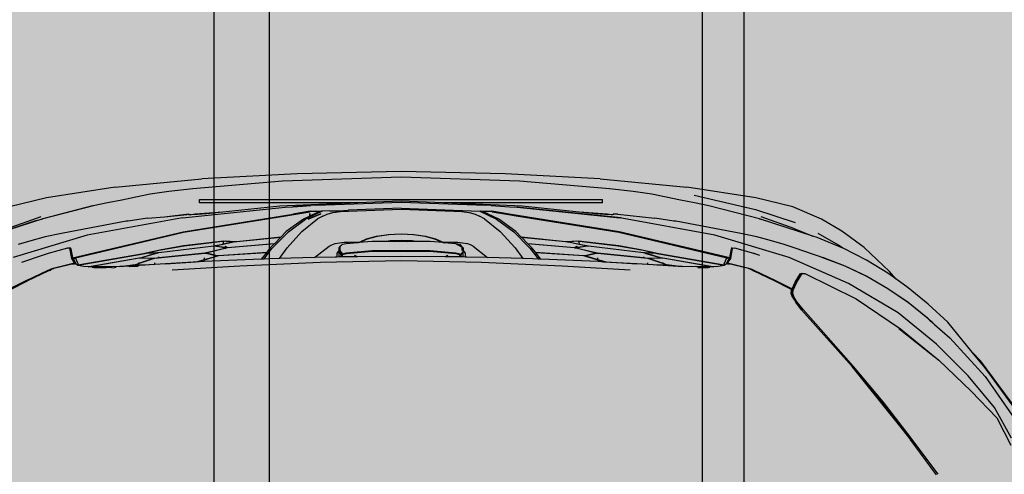
# Model space of a CAD drawing. Units: inches. Extents: x 1884 to 2398, y 474 to 1488.
# Tile 29 of 39: x 2306 to 2356, y 737 to 761. Entities that reach past the tile are written whole.
import ezdxf

# ---------------------------------------------------------------- set-up
doc = ezdxf.new("R2010")
doc.units = ezdxf.units.IN
doc.header["$MEASUREMENT"] = 0
doc.layers.get('0').update_dxf_attribs({"color": 250})
doc.layers.add('A-ANNO-DIMS', color=2, linetype='Continuous', lineweight=18)
doc.layers.add('C-VEHI', color=8, linetype='Continuous', lineweight=18)
doc.layers.add('Edges', color=250, linetype='Continuous')
doc.layers.add('L-PVMT-PATT', color=9, linetype='Continuous', lineweight=13, true_color=0xc7c8ca)
doc.styles.get("Standard").update_dxf_attribs({"font": 'arial.ttf'})
doc.dimstyles.get("Standard").update_dxf_attribs({"dimtxt": 7, "dimasz": 0.18, "dimexe": 0.18, "dimexo": 0.0625, "dimgap": 0.09, "dimtad": 0, "dimtih": 1, "dimtoh": 1, "dimzin": 0, "dimdsep": 46, "dimlunit": 3, "dimtxsty": 'Standard', "dimcen": 0.09, "dimadec": 0, "dimazin": 0, "dimtfac": 1, "dimtofl": 0, "dimtmove": 0, "dimatfit": 3, "dimfxl": 1, "dimtolj": 1, "dimtzin": 0, "dimarcsym": 0})

# ---------------------------------------------------------------- blocks, each defined once
blk = doc.blocks.new('Nissan Qashqai pl')
at = {"layer": 'Edges'}
for p, q in [((7.6024, 12.7221), (7.5387, 12.6759)), ((7.5946, 12.718), (7.5304, 12.6704)), ((7.5501, 12.6757), (7.6051, 12.7139)), ((7.6295, 12.7097), (7.59, 12.6877)), ((7.6032, 12.6908), (7.6386, 12.7089)), ((7.59, 12.6877), (7.5492, 12.654)), ((7.5687, 12.6579), (7.6032, 12.6908)), ((7.5501, 12.6757), (7.5001, 12.6302)), ((7.5387, 12.6759), (7.5184, 12.6591)), ((7.5184, 12.6591), (7.5304, 12.6704)), ((7.5184, 12.6591), (7.4801, 12.6274)), ((7.5289, 12.6158), (7.5687, 12.6579)), ((7.5492, 12.654), (7.531, 12.6359)), ((7.4827, 12.6103), (7.5001, 12.6302)), ((7.531, 12.6359), (7.5081, 12.6131)), ((7.531, 12.6359), (7.5301, 12.6353)), ((7.4801, 12.6274), (7.4565, 12.6023)), ((7.5081, 12.6131), (7.4679, 12.5634)), ((7.4744, 12.6015), (7.4804, 12.6079)), ((7.4762, 12.6028), (7.478, 12.6049)), ((7.4804, 12.6079), (7.478, 12.6049)), ((7.478, 12.6049), (7.479, 12.6061)), ((7.479, 12.6061), (7.4815, 12.6089)), ((7.479, 12.6061), (7.4801, 12.6074)), ((7.4801, 12.6074), (7.4804, 12.6079)), ((7.4804, 12.6079), (7.4807, 12.6082)), ((7.4804, 12.6079), (7.4804, 12.6079)), ((7.4807, 12.6082), (7.4821, 12.6097)), ((7.4815, 12.6089), (7.4821, 12.6097)), ((7.4821, 12.6097), (7.4827, 12.6103)), ((7.4882, 12.5645), (7.5243, 12.6101)), ((7.4884, 12.5664), (7.5289, 12.6158)), ((7.5243, 12.6101), (7.5286, 12.6146)), ((7.676, 12.6152), (7.6296, 12.5803)), ((7.6769, 12.6129), (7.6306, 12.5791)), ((7.4565, 12.6023), (7.4354, 12.5766)), ((7.4542, 12.5765), (7.4744, 12.6015)), ((7.475, 12.6016), (7.4549, 12.5767)), ((7.4762, 12.6028), (7.475, 12.6016)), ((7.4752, 12.6016), (7.4762, 12.6028)), ((7.6296, 12.5803), (7.5827, 12.5441)), ((7.6301, 12.5787), (7.618, 12.5691)), ((7.6306, 12.5791), (7.6301, 12.5787)), ((7.4354, 12.5766), (7.4239, 12.5604)), ((7.4363, 12.5502), (7.4542, 12.5765)), ((7.4549, 12.5767), (7.4369, 12.5504)), ((7.4498, 12.5093), (7.4884, 12.5664)), ((7.618, 12.5691), (7.5829, 12.5411)), ((7.618, 12.5691), (7.584, 12.5429)), ((7.4239, 12.5604), (7.4147, 12.5524)), ((7.4239, 12.5604), (7.4166, 12.5503)), ((7.4679, 12.5634), (7.4302, 12.4993)), ((7.4147, 12.5524), (7.3837, 12.5197)), ((7.4166, 12.5503), (7.3997, 12.5227)), ((7.4205, 12.5229), (7.4363, 12.5502)), ((7.4369, 12.5504), (7.4211, 12.5232)), ((7.5827, 12.5441), (7.5369, 12.5057)), ((7.584, 12.5429), (7.5568, 12.5201)), ((7.5829, 12.5411), (7.5568, 12.5201)), ((7.3837, 12.5197), (7.3624, 12.4907)), ((7.3997, 12.5227), (7.3845, 12.4925)), ((7.4071, 12.4948), (7.4205, 12.5229)), ((7.4211, 12.5232), (7.4078, 12.4951)), ((7.5568, 12.5201), (7.5371, 12.5042)), ((7.4172, 12.4431), (7.4498, 12.5093)), ((7.5369, 12.5057), (7.4635, 12.4408)), ((7.4638, 12.439), (7.5371, 12.5042)), ((7.3624, 12.4907), (7.347, 12.4644)), ((7.3843, 12.492), (7.3707, 12.4592)), ((7.3843, 12.492), (7.3805, 12.4866)), ((7.3845, 12.4925), (7.3843, 12.492)), ((7.3962, 12.466), (7.4071, 12.4948)), ((7.4302, 12.4993), (7.3963, 12.4227)), ((7.4078, 12.4951), (7.3969, 12.4665)), ((7.3805, 12.4866), (7.3655, 12.4604)), ((7.347, 12.4644), (7.3309, 12.4276)), ((7.3965, 12.4655), (7.3951, 12.462)), ((7.3965, 12.4655), (7.3962, 12.466)), ((7.3969, 12.4665), (7.3965, 12.4655)), ((7.3968, 12.4649), (7.3967, 12.4651)), ((7.3688, 12.4532), (7.3467, 12.3846)), ((7.3596, 12.4302), (7.3688, 12.4532)), ((7.3707, 12.4592), (7.3688, 12.4532)), ((7.3925, 12.4542), (7.3845, 12.4306)), ((7.3938, 12.4583), (7.3925, 12.4542)), ((7.3951, 12.462), (7.3938, 12.4583)), ((7.4167, 12.4393), (7.4169, 12.4406)), ((7.4167, 12.4393), (7.4172, 12.4395)), ((7.417, 12.4377), (7.4167, 12.4393)), ((7.4169, 12.4412), (7.4172, 12.4431)), ((7.4169, 12.4406), (7.4172, 12.4423)), ((7.4169, 12.4406), (7.4169, 12.4412)), ((7.4169, 12.4398), (7.4169, 12.4406)), ((7.4282, 12.4328), (7.4169, 12.4398)), ((7.4172, 12.4395), (7.4169, 12.4398)), ((7.4172, 12.4423), (7.4174, 12.4429)), ((7.4183, 12.4382), (7.4172, 12.4395)), ((7.4175, 12.4429), (7.4174, 12.4429)), ((7.4635, 12.4408), (7.4541, 12.4333)), ((7.4638, 12.439), (7.4541, 12.4313)), ((7.3309, 12.4276), (7.3193, 12.3797)), ((7.3345, 12.3793), (7.3514, 12.4308)), ((7.3596, 12.4302), (7.344, 12.3869)), ((7.3845, 12.4306), (7.3799, 12.4164)), ((7.4283, 12.4307), (7.417, 12.4377)), ((7.4183, 12.4382), (7.4296, 12.4312)), ((7.4255, 12.4044), (7.4367, 12.4268)), ((7.4387, 12.428), (7.4282, 12.4328)), ((7.4359, 12.4272), (7.4283, 12.4307)), ((7.4383, 12.4272), (7.4296, 12.4312)), ((7.4367, 12.4268), (7.4359, 12.4272)), ((7.4378, 12.4261), (7.4365, 12.4235)), ((7.4367, 12.4268), (7.4383, 12.4272)), ((7.4379, 12.4263), (7.4378, 12.4261)), ((7.4379, 12.4263), (7.4383, 12.4272)), ((7.4379, 12.4263), (7.4389, 12.4269)), ((7.4384, 12.426), (7.4379, 12.4263)), ((7.4384, 12.426), (7.438, 12.4251)), ((7.4383, 12.4272), (7.4389, 12.4269)), ((7.4389, 12.4269), (7.4384, 12.426)), ((7.4387, 12.4259), (7.4384, 12.426)), ((7.4431, 12.4276), (7.4387, 12.428)), ((7.443, 12.4254), (7.4387, 12.4259)), ((7.44, 12.4264), (7.4389, 12.4269)), ((7.44, 12.4264), (7.4442, 12.4258)), ((7.4477, 12.427), (7.443, 12.4254)), ((7.4479, 12.4293), (7.4431, 12.4276)), ((7.4442, 12.4258), (7.4477, 12.427)), ((7.4477, 12.427), (7.4541, 12.4313)), ((7.4541, 12.4333), (7.4479, 12.4293)), ((7.3963, 12.4227), (7.3676, 12.3269)), ((7.3799, 12.4164), (7.375, 12.4)), ((7.4365, 12.4235), (7.4267, 12.4041)), ((7.4365, 12.4235), (7.4365, 12.4235)), ((7.4131, 12.3783), (7.4255, 12.4044)), ((7.4267, 12.4041), (7.4139, 12.3778)), ((7.3467, 12.3846), (7.3489, 12.3925)), ((7.375, 12.4), (7.3699, 12.3813)), ((7.3193, 12.3797), (7.3059, 12.291)), ((7.3161, 12.3001), (7.3345, 12.3793)), ((7.3467, 12.3846), (7.33, 12.3192)), ((7.3699, 12.3813), (7.3653, 12.3604)), ((7.3913, 12.3774), (7.3844, 12.3526)), ((7.3913, 12.3774), (7.3914, 12.3775)), ((7.3925, 12.3813), (7.3914, 12.3775)), ((7.3937, 12.3851), (7.3925, 12.3813)), ((7.4115, 12.3746), (7.4131, 12.3783)), ((7.4139, 12.3778), (7.4122, 12.3742)), ((7.4133, 12.3759), (7.4142, 12.3776)), ((7.4033, 12.3435), (7.4101, 12.3708)), ((7.4108, 12.3703), (7.4042, 12.3435)), ((7.4101, 12.3708), (7.4115, 12.3746)), ((7.4122, 12.3742), (7.4108, 12.3703)), ((7.3653, 12.3604), (7.3497, 12.2767)), ((7.3841, 12.3485), (7.3844, 12.3526)), ((7.3971, 12.3461), (7.3635, 12.2033)), ((7.364, 12.2029), (7.3968, 12.3424)), ((7.3846, 12.3495), (7.3841, 12.3485)), ((7.3841, 12.3485), (7.3853, 12.3483)), ((7.3846, 12.3495), (7.3976, 12.347)), ((7.3971, 12.3461), (7.3853, 12.3483)), ((7.3916, 12.2547), (7.4062, 12.3389)), ((7.4065, 12.3392), (7.3917, 12.2547)), ((7.3968, 12.3424), (7.398, 12.3449)), ((7.4046, 12.3389), (7.3968, 12.3424)), ((7.3983, 12.3458), (7.3971, 12.3461)), ((7.3976, 12.347), (7.4026, 12.3439)), ((7.398, 12.3449), (7.3999, 12.344)), ((7.398, 12.3449), (7.4012, 12.3441)), ((7.4012, 12.3441), (7.3983, 12.3458)), ((7.3999, 12.344), (7.4051, 12.3415)), ((7.3999, 12.344), (7.4048, 12.3417)), ((7.4033, 12.3427), (7.4012, 12.3441)), ((7.4012, 12.3441), (7.4015, 12.344)), ((7.4015, 12.344), (7.4028, 12.3437)), ((7.4026, 12.3439), (7.4033, 12.3435)), ((7.4033, 12.3435), (7.4042, 12.3422)), ((7.4042, 12.3422), (7.4033, 12.3427)), ((7.4042, 12.3435), (7.404, 12.3429)), ((7.404, 12.3429), (7.4043, 12.3428)), ((7.404, 12.3429), (7.4043, 12.3425)), ((7.4041, 12.3435), (7.4042, 12.3435)), ((7.4042, 12.3435), (7.4045, 12.3434)), ((7.4042, 12.3422), (7.4043, 12.3425)), ((7.4044, 12.3422), (7.4042, 12.3422)), ((7.4043, 12.3428), (7.4045, 12.3434)), ((7.4043, 12.3428), (7.4046, 12.3425)), ((7.4043, 12.3425), (7.4043, 12.3428)), ((7.4043, 12.3425), (7.4044, 12.3422)), ((7.4044, 12.3422), (7.4046, 12.3419)), ((7.4046, 12.3422), (7.4044, 12.3422)), ((7.4045, 12.3434), (7.405, 12.3456)), ((7.4045, 12.3434), (7.4048, 12.3433)), ((7.4046, 12.3425), (7.4047, 12.3424)), ((7.4047, 12.3424), (7.4046, 12.3422)), ((7.4046, 12.3422), (7.4046, 12.3419)), ((7.4048, 12.3422), (7.4046, 12.3422)), ((7.4046, 12.3419), (7.405, 12.3419)), ((7.4048, 12.3417), (7.4046, 12.3419)), ((7.4046, 12.3389), (7.4062, 12.3389)), ((7.4047, 12.3424), (7.4048, 12.3422)), ((7.4048, 12.3422), (7.405, 12.3419)), ((7.4048, 12.3417), (7.4052, 12.3416)), ((7.4051, 12.3415), (7.4048, 12.3417)), ((7.405, 12.3419), (7.4052, 12.3416)), ((7.4051, 12.3415), (7.4052, 12.3415)), ((7.4052, 12.3416), (7.4052, 12.3415)), ((7.4052, 12.3415), (7.4063, 12.3395)), ((7.4062, 12.3389), (7.4063, 12.3395)), ((7.4063, 12.3395), (7.4065, 12.3392)), ((7.4065, 12.3392), (7.4066, 12.3389)), ((7.4066, 12.3389), (7.408, 12.3313)), ((7.3676, 12.3269), (7.3455, 12.2042)), ((7.3971, 12.2599), (7.4083, 12.3258)), ((7.4084, 12.3244), (7.3975, 12.2599)), ((7.408, 12.3313), (7.4083, 12.3258)), ((7.4083, 12.3258), (7.4084, 12.3244)), ((7.4084, 12.3244), (7.4087, 12.3195)), ((7.33, 12.3192), (7.3261, 12.3009)), ((7.4087, 12.3195), (7.4087, 12.3037)), ((7.4092, 12.3184), (7.4091, 12.3206)), ((7.4092, 12.305), (7.4092, 12.3184)), ((7.3261, 12.3009), (7.3223, 12.2825)), ((7.4087, 12.3037), (7.4081, 12.2848)), ((7.2951, 12.1791), (7.3059, 12.291)), ((7.3223, 12.2825), (7.3186, 12.2641)), ((7.3494, 12.2741), (7.3457, 12.2495)), ((7.3498, 12.2768), (7.3494, 12.2741)), ((7.3497, 12.2767), (7.3494, 12.2741)), ((7.4054, 12.2651), (7.4081, 12.2848)), ((7.4079, 12.2798), (7.4059, 12.2651)), ((7.4079, 12.2798), (7.4069, 12.2598)), ((7.4081, 12.2838), (7.4079, 12.2798)), ((7.4081, 12.2848), (7.4081, 12.2838)), ((7.3186, 12.2641), (7.3149, 12.2457)), ((7.4048, 12.2612), (7.3982, 12.2419)), ((7.4038, 12.2599), (7.4049, 12.2631)), ((7.4053, 12.2622), (7.4048, 12.2612)), ((7.4049, 12.2631), (7.4054, 12.2651)), ((7.4053, 12.2612), (7.4053, 12.2622)), ((7.4061, 12.2473), (7.4053, 12.2612)), ((7.4059, 12.2618), (7.4056, 12.2621)), ((7.4059, 12.2651), (7.4058, 12.2632)), ((7.4058, 12.2632), (7.4059, 12.2618)), ((7.4059, 12.2618), (7.4064, 12.2523)), ((7.3407, 12.2016), (7.3457, 12.2495)), ((7.3909, 12.2508), (7.3864, 12.231)), ((7.3869, 12.2347), (7.3912, 12.2527)), ((7.3901, 12.2368), (7.391, 12.2507)), ((7.3914, 12.2527), (7.3906, 12.2386)), ((7.3908, 12.2366), (7.3965, 12.256)), ((7.3911, 12.2518), (7.3909, 12.2508)), ((7.391, 12.2387), (7.3967, 12.2579)), ((7.391, 12.2507), (7.3911, 12.2518)), ((7.3912, 12.2517), (7.3911, 12.2518)), ((7.3912, 12.2527), (7.3916, 12.2547)), ((7.3917, 12.2547), (7.3914, 12.2527)), ((7.3969, 12.257), (7.3965, 12.256)), ((7.3967, 12.2579), (7.3971, 12.2599)), ((7.3968, 12.2559), (7.3969, 12.257)), ((7.3972, 12.2421), (7.3968, 12.2559)), ((7.3975, 12.2599), (7.3973, 12.258)), ((7.3973, 12.258), (7.3977, 12.2439)), ((7.3983, 12.244), (7.4038, 12.2599)), ((7.4028, 12.2599), (7.4038, 12.2599)), ((7.4064, 12.2523), (7.4061, 12.2473)), ((7.4069, 12.2598), (7.4064, 12.2523)), ((7.3149, 12.2457), (7.3113, 12.2217)), ((7.3899, 12.2348), (7.3901, 12.2368)), ((7.3908, 12.2366), (7.3903, 12.2347)), ((7.3906, 12.2386), (7.3907, 12.2376)), ((7.3907, 12.2376), (7.391, 12.2387)), ((7.3977, 12.24), (7.3911, 12.1755)), ((7.3966, 12.2348), (7.3972, 12.24)), ((7.3972, 12.24), (7.3972, 12.2421)), ((7.3977, 12.2439), (7.398, 12.2429)), ((7.3982, 12.2419), (7.3977, 12.24)), ((7.398, 12.2429), (7.3983, 12.244)), ((7.4032, 12.24), (7.4057, 12.24)), ((7.4057, 12.24), (7.4048, 12.2262)), ((7.4061, 12.2472), (7.4057, 12.24)), ((7.4061, 12.2472), (7.4061, 12.2473)), ((7.3813, 12.2021), (7.3869, 12.2347)), ((7.3815, 12.1638), (7.3899, 12.2348)), ((7.3864, 12.231), (7.3815, 12.2029)), ((7.3903, 12.2347), (7.382, 12.1639)), ((7.3905, 12.1754), (7.3966, 12.2347)), ((7.3957, 12.2348), (7.3966, 12.2348)), ((7.3957, 12.2347), (7.3966, 12.2347)), ((7.3966, 12.2347), (7.3966, 12.2348)), ((7.4022, 12.187), (7.4048, 12.2262)), ((7.4048, 12.2262), (7.4023, 12.1836)), ((7.3113, 12.2217), (7.3078, 12.191)), ((7.4072, 12.1299), (7.4124, 12.2176)), ((7.3455, 12.2062), (7.3317, 12.0717)), ((7.3317, 12.0717), (7.3455, 12.2042)), ((7.3407, 12.2016), (7.34, 12.1962)), ((7.3403, 12.1981), (7.3407, 12.2016)), ((7.3635, 12.2033), (7.3405, 12.0616)), ((7.3426, 12.0707), (7.364, 12.2029)), ((7.375, 12.1484), (7.3813, 12.2021)), ((7.3815, 12.2029), (7.3756, 12.1509)), ((7.3078, 12.191), (7.298, 12.075)), ((7.3407, 12.1879), (7.3378, 12.1521)), ((7.34, 12.1962), (7.3401, 12.1962)), ((7.341, 12.1848), (7.34, 12.1731)), ((7.3401, 12.1962), (7.341, 12.1962)), ((7.3413, 12.1933), (7.3407, 12.1879)), ((7.341, 12.1962), (7.3414, 12.1962)), ((7.341, 12.1962), (7.341, 12.1962)), ((7.3414, 12.1962), (7.341, 12.1962)), ((7.341, 12.1962), (7.3413, 12.1933)), ((7.3413, 12.1931), (7.341, 12.1848)), ((7.3415, 12.1954), (7.3413, 12.1933)), ((7.3413, 12.1933), (7.3413, 12.1931)), ((7.399, 12.1756), (7.4017, 12.185)), ((7.4017, 12.185), (7.4022, 12.187)), ((7.2951, 12.1791), (7.2884, 12.0562)), ((7.3261, 12.1821), (7.3216, 12.1821)), ((7.3216, 11.6621), (7.3216, 12.1821)), ((7.3261, 12.1821), (7.3261, 11.9779)), ((7.34, 12.1731), (7.3378, 12.1521)), ((7.3877, 12.1639), (7.3901, 12.1734)), ((7.3901, 12.1734), (7.3905, 12.1754)), ((7.3907, 12.1727), (7.3903, 12.1716)), ((7.3909, 12.1716), (7.3907, 12.1727)), ((7.3911, 12.1755), (7.3913, 12.1737)), ((7.3913, 12.1737), (7.3943, 12.1614)), ((7.3949, 12.1616), (7.399, 12.1756)), ((7.4021, 12.1833), (7.3951, 12.1606)), ((7.3967, 12.1756), (7.399, 12.1756)), ((7.4018, 12.1764), (7.3986, 12.1025)), ((7.4023, 12.1836), (7.4018, 12.1764)), ((7.4023, 12.1836), (7.4021, 12.1833)), ((7.3813, 12.1599), (7.3763, 12.1361)), ((7.3792, 12.1518), (7.3812, 12.1619)), ((7.3812, 12.1619), (7.3815, 12.1638)), ((7.3815, 12.161), (7.3813, 12.1599)), ((7.3817, 12.16), (7.3815, 12.161)), ((7.3832, 12.1493), (7.3817, 12.16)), ((7.382, 12.1639), (7.382, 12.1619)), ((7.382, 12.1619), (7.3838, 12.1497)), ((7.3843, 12.1498), (7.3877, 12.1639)), ((7.3903, 12.1716), (7.3844, 12.1479)), ((7.3877, 12.1639), (7.3874, 12.1639)), ((7.3939, 12.1596), (7.3909, 12.1716)), ((7.3941, 12.1576), (7.3939, 12.1596)), ((7.3943, 12.1614), (7.3947, 12.1605)), ((7.3951, 12.1606), (7.3945, 12.1577)), ((7.3947, 12.1605), (7.3949, 12.1616)), ((7.3378, 12.1521), (7.3302, 12.0785)), ((7.376, 12.136), (7.375, 12.1484)), ((7.3756, 12.1509), (7.3792, 12.1518)), ((7.3756, 12.1509), (7.3762, 12.138)), ((7.3764, 12.138), (7.3792, 12.1518)), ((7.3832, 12.1493), (7.3824, 12.1487)), ((7.3824, 12.1487), (7.3832, 12.1492)), ((7.3836, 12.1459), (7.3824, 12.1487)), ((7.3824, 12.1487), (7.3835, 12.1468)), ((7.3838, 12.1497), (7.3832, 12.1493)), ((7.3832, 12.1492), (7.3837, 12.1495)), ((7.3832, 12.1492), (7.3832, 12.1493)), ((7.3836, 12.1459), (7.3835, 12.1468)), ((7.3835, 12.1468), (7.384, 12.1459)), ((7.3837, 12.1495), (7.3843, 12.1498)), ((7.3837, 12.1495), (7.3838, 12.1497)), ((7.384, 12.1459), (7.3842, 12.1495)), ((7.3844, 12.1479), (7.384, 12.1459)), ((7.3842, 12.1495), (7.3843, 12.1498)), ((7.3843, 12.1495), (7.3842, 12.1495)), ((7.3896, 12.0954), (7.3941, 12.1576)), ((7.3945, 12.1577), (7.3903, 12.0959)), ((7.3701, 12.0771), (7.3759, 12.1341)), ((7.3761, 12.1341), (7.3704, 12.0773)), ((7.3759, 12.1341), (7.376, 12.136)), ((7.3763, 12.1361), (7.3761, 12.1341)), ((7.3762, 12.137), (7.3764, 12.138)), ((7.3762, 12.138), (7.3762, 12.137)), ((7.3764, 12.1371), (7.3762, 12.137)), ((7.3783, 12.0852), (7.3836, 12.1459)), ((7.384, 12.1459), (7.3788, 12.0857)), ((7.4025, 12.026), (7.4072, 12.1299)), ((7.3845, 12.0883), (7.3985, 12.0993)), ((7.3903, 12.0959), (7.3896, 12.0954)), ((7.3986, 12.1025), (7.3903, 12.0959)), ((7.3985, 12.0993), (7.3982, 12.092)), ((7.3986, 12.1025), (7.3985, 12.0993)), ((7.3633, 12.0674), (7.3845, 12.0883)), ((7.3783, 12.0852), (7.3704, 12.0773)), ((7.3788, 12.0857), (7.3783, 12.0852)), ((7.3841, 12.091), (7.3788, 12.0857)), ((7.3896, 12.0954), (7.3841, 12.091)), ((7.3982, 12.092), (7.3978, 12.0791)), ((7.298, 12.075), (7.2928, 11.9221)), ((7.3302, 12.0785), (7.3261, 11.9779)), ((7.3309, 12.0619), (7.3317, 12.0717)), ((7.341, 12.0605), (7.3426, 12.0707)), ((7.3631, 12.0701), (7.3469, 12.0481)), ((7.3701, 12.0771), (7.3631, 12.0701)), ((7.3704, 12.0773), (7.3701, 12.0771)), ((7.3842, 12.0693), (7.3978, 12.0791)), ((7.3978, 12.0791), (7.3966, 12.0338)), ((7.3294, 12.0385), (7.3309, 12.0619)), ((7.3405, 12.0616), (7.3369, 12.0394)), ((7.3377, 12.0398), (7.341, 12.0605)), ((7.3471, 12.0454), (7.3633, 12.0674)), ((7.363, 12.0501), (7.3842, 12.0693)), ((7.2884, 12.0562), (7.2857, 11.9221)), ((7.3365, 12.0237), (7.3471, 12.0454)), ((7.3469, 12.0481), (7.3402, 12.0337)), ((7.3468, 12.0299), (7.363, 12.0501)), ((7.3294, 12.0385), (7.3291, 12.0316)), ((7.3362, 12.0248), (7.3365, 12.0321)), ((7.3365, 12.0321), (7.3369, 12.0394)), ((7.3377, 12.0398), (7.3369, 12.0328)), ((7.3369, 12.0287), (7.3369, 12.0328)), ((7.3402, 12.0337), (7.338, 12.0291)), ((7.3387, 12.0332), (7.3402, 12.0337)), ((7.3818, 12.0151), (7.3966, 12.0338)), ((7.3966, 12.0338), (7.3959, 12.0071)), ((7.3251, 11.9221), (7.3291, 12.0316)), ((7.3329, 11.9221), (7.3365, 12.0237)), ((7.3362, 12.0248), (7.3366, 12.0246)), ((7.3365, 12.0237), (7.3362, 12.0248)), ((7.338, 12.0291), (7.3369, 12.0287)), ((7.3374, 12.0276), (7.3369, 12.0287)), ((7.338, 12.0291), (7.3374, 12.0276)), ((7.3407, 12.0176), (7.3432, 12.0231)), ((7.3468, 12.0299), (7.3432, 12.0231)), ((7.4002, 11.9221), (7.4025, 12.026)), ((7.3373, 12.0004), (7.3386, 12.01)), ((7.3386, 12.01), (7.3407, 12.0176)), ((7.3775, 12.0015), (7.3786, 12.007)), ((7.3801, 12.0115), (7.3786, 12.007)), ((7.3818, 12.0151), (7.3801, 12.0115)), ((7.3959, 12.0071), (7.3959, 12.0051)), ((7.3367, 11.99), (7.3373, 12.0004)), ((7.3765, 11.989), (7.3768, 11.9954)), ((7.3768, 11.9954), (7.3775, 12.0015)), ((7.3798, 11.9983), (7.3787, 11.9928)), ((7.3787, 11.9928), (7.38, 11.9953)), ((7.3808, 11.9993), (7.3798, 11.9983)), ((7.3807, 11.9991), (7.3798, 11.9983)), ((7.38, 11.9953), (7.383, 12.0011)), ((7.3807, 11.9991), (7.3808, 11.9993)), ((7.381, 11.9993), (7.3807, 11.9991)), ((7.3808, 11.9993), (7.384, 12.0021)), ((7.381, 11.9993), (7.3808, 11.9993)), ((7.383, 12.0011), (7.381, 11.9993)), ((7.3866, 12.0011), (7.383, 12.0011)), ((7.384, 12.0021), (7.387, 12.0021)), ((7.3868, 12.002), (7.3866, 12.0011)), ((7.3875, 12.0011), (7.3866, 12.0011)), ((7.387, 12.0021), (7.3868, 12.002)), ((7.3909, 12.0051), (7.387, 12.0021)), ((7.387, 12.0021), (7.3885, 12.0021)), ((7.3885, 12.0021), (7.3925, 11.9993)), ((7.3955, 12.0021), (7.3885, 12.0021)), ((7.3904, 11.9928), (7.3916, 11.9983)), ((7.3956, 12.0051), (7.3909, 12.0051)), ((7.3929, 11.9981), (7.3917, 11.9926)), ((7.3925, 11.9993), (7.3958, 11.9993)), ((7.3925, 11.9993), (7.3929, 11.9981)), ((7.3958, 11.9981), (7.3929, 11.9981)), ((7.3955, 12.0021), (7.3958, 12.0018)), ((7.3959, 12.0049), (7.3956, 12.0051)), ((7.3959, 12.0051), (7.3956, 12.0051)), ((7.3958, 11.9981), (7.3956, 11.9801)), ((7.3959, 12.0049), (7.3958, 12.0018)), ((7.3958, 12.0018), (7.3958, 11.9993)), ((7.3958, 11.9993), (7.3958, 11.9981)), ((7.3959, 12.0051), (7.3959, 12.0049)), ((7.3343, 11.9221), (7.3367, 11.99)), ((7.3761, 11.9751), (7.3765, 11.989)), ((7.3787, 11.9928), (7.3774, 11.9778)), ((7.3876, 11.9595), (7.3904, 11.9928)), ((7.3917, 11.9926), (7.3889, 11.9594)), ((7.3938, 11.9823), (7.3956, 11.9801)), ((7.3261, 11.9764), (7.3238, 11.9221)), ((7.3261, 11.9764), (7.3261, 11.9779)), ((7.3724, 11.9667), (7.3761, 11.9751)), ((7.3771, 11.9757), (7.3727, 11.9658)), ((7.3773, 11.9759), (7.3759, 11.9595)), ((7.3761, 11.9751), (7.3769, 11.9767)), ((7.3769, 11.9767), (7.3771, 11.977)), ((7.3774, 11.9778), (7.3771, 11.9771)), ((7.3771, 11.9771), (7.3774, 11.9774)), ((7.3771, 11.9771), (7.3771, 11.977)), ((7.3773, 11.9759), (7.3771, 11.9757)), ((7.3774, 11.9774), (7.3773, 11.9759)), ((7.3774, 11.9774), (7.3774, 11.9778)), ((7.3956, 11.9788), (7.3938, 11.981)), ((7.3956, 11.9788), (7.3951, 11.9221)), ((7.3956, 11.9801), (7.3956, 11.9788)), ((7.369, 11.9536), (7.3724, 11.9667)), ((7.3727, 11.9658), (7.3693, 11.953)), ((7.3759, 11.9595), (7.3759, 11.9417)), ((7.3876, 11.8847), (7.3876, 11.9595)), ((7.3889, 11.9594), (7.3889, 11.8848)), ((7.3668, 11.9384), (7.369, 11.9536)), ((7.3693, 11.953), (7.3672, 11.9381)), ((7.3661, 11.9221), (7.3668, 11.9384)), ((7.3672, 11.9381), (7.3665, 11.9221)), ((7.3751, 11.9363), (7.3745, 11.9221)), ((7.3759, 11.9417), (7.3751, 11.9363)), ((7.3759, 11.9417), (7.3759, 11.9303)), ((7.2857, 11.9221), (7.2884, 11.7879)), ((7.2928, 11.9221), (7.298, 11.7692)), ((7.3238, 11.9221), (7.3261, 11.8662)), ((7.3291, 11.8126), (7.3251, 11.9221)), ((7.3329, 11.9221), (7.3354, 11.8539)), ((7.3367, 11.8541), (7.3343, 11.9221)), ((7.3668, 11.9057), (7.3661, 11.9221)), ((7.3665, 11.9221), (7.3672, 11.9061)), ((7.3745, 11.9221), (7.3751, 11.9078)), ((7.3755, 11.9221), (7.3759, 11.9303)), ((7.3759, 11.9139), (7.3755, 11.9221)), ((7.3759, 11.9303), (7.3759, 11.9139)), ((7.3951, 11.9221), (7.3956, 11.8653)), ((7.4025, 11.8181), (7.4002, 11.9221)), ((7.369, 11.8905), (7.3668, 11.9057)), ((7.3672, 11.9061), (7.3693, 11.8911)), ((7.3751, 11.9078), (7.3759, 11.9025)), ((7.3759, 11.9139), (7.3759, 11.9025)), ((7.3759, 11.9025), (7.3759, 11.8847)), ((7.3724, 11.8775), (7.369, 11.8905)), ((7.3693, 11.8911), (7.3727, 11.8783)), ((7.3759, 11.8847), (7.3773, 11.8682)), ((7.3904, 11.8513), (7.3876, 11.8847)), ((7.3889, 11.8848), (7.3917, 11.8516)), ((7.3761, 11.8691), (7.3724, 11.8775)), ((7.3727, 11.8783), (7.3771, 11.8685)), ((7.3765, 11.8551), (7.3761, 11.8691)), ((7.3769, 11.8674), (7.3761, 11.8691)), ((7.3771, 11.8671), (7.3769, 11.8674)), ((7.3771, 11.8685), (7.3773, 11.8682)), ((7.3771, 11.8671), (7.3771, 11.8671)), ((7.3771, 11.8671), (7.3774, 11.8664)), ((7.3774, 11.8668), (7.3771, 11.8671)), ((7.3773, 11.8682), (7.3774, 11.8668)), ((7.3261, 11.8662), (7.3302, 11.7656)), ((7.3261, 11.8662), (7.3261, 11.6621)), ((7.3373, 11.8438), (7.3367, 11.8541)), ((7.3768, 11.8488), (7.3765, 11.8551)), ((7.3774, 11.8668), (7.3774, 11.8664)), ((7.3774, 11.8664), (7.3787, 11.8513)), ((7.3938, 11.8632), (7.3956, 11.8653)), ((7.3956, 11.864), (7.3938, 11.8619)), ((7.3956, 11.8653), (7.3956, 11.864)), ((7.3956, 11.864), (7.3958, 11.8461)), ((7.3361, 11.8416), (7.3354, 11.8539)), ((7.3362, 11.8301), (7.3361, 11.8416)), ((7.3386, 11.8342), (7.3373, 11.8438)), ((7.3775, 11.8427), (7.3768, 11.8488)), ((7.3786, 11.8372), (7.3775, 11.8427)), ((7.3787, 11.8513), (7.3798, 11.8459)), ((7.3798, 11.8459), (7.3808, 11.8448)), ((7.3808, 11.8448), (7.3807, 11.8451)), ((7.3808, 11.8448), (7.381, 11.8448)), ((7.384, 11.8421), (7.3808, 11.8448)), ((7.383, 11.8431), (7.3875, 11.8431)), ((7.387, 11.8421), (7.384, 11.8421)), ((7.387, 11.8421), (7.3909, 11.8391)), ((7.3885, 11.8421), (7.387, 11.8421)), ((7.3875, 11.8431), (7.3916, 11.8459)), ((7.3925, 11.8448), (7.3885, 11.8421)), ((7.3955, 11.8421), (7.3885, 11.8421)), ((7.3916, 11.8459), (7.3904, 11.8513)), ((7.3917, 11.8516), (7.3929, 11.8461)), ((7.3929, 11.8461), (7.3925, 11.8448)), ((7.3958, 11.8448), (7.3925, 11.8448)), ((7.3929, 11.8461), (7.3958, 11.8461)), ((7.3958, 11.8423), (7.3955, 11.8421)), ((7.3958, 11.8461), (7.3958, 11.8448)), ((7.3958, 11.8448), (7.3958, 11.8423)), ((7.3958, 11.8423), (7.3959, 11.8392)), ((7.3362, 11.8301), (7.3365, 11.8204)), ((7.3407, 11.8266), (7.3386, 11.8342)), ((7.3801, 11.8327), (7.3786, 11.8372)), ((7.3818, 11.8291), (7.3801, 11.8327)), ((7.3966, 11.8103), (7.3818, 11.8291)), ((7.3909, 11.8391), (7.3956, 11.8391)), ((7.3956, 11.8391), (7.3959, 11.8392)), ((7.3956, 11.8391), (7.3959, 11.8391)), ((7.3959, 11.8392), (7.3959, 11.8391)), ((7.3959, 11.8391), (7.3959, 11.8371)), ((7.3959, 11.8371), (7.3966, 11.8103)), ((7.3362, 11.8194), (7.3365, 11.8204)), ((7.3367, 11.8196), (7.3362, 11.8194)), ((7.3365, 11.812), (7.3362, 11.8194)), ((7.3365, 11.8204), (7.3471, 11.7987)), ((7.3369, 11.8155), (7.3374, 11.8165)), ((7.3374, 11.8165), (7.338, 11.8151)), ((7.3401, 11.8186), (7.3431, 11.8112)), ((7.347, 11.8021), (7.3401, 11.8186)), ((7.3432, 11.821), (7.3407, 11.8266)), ((7.3432, 11.821), (7.3468, 11.8142)), ((7.4072, 11.7142), (7.4025, 11.8181)), ((7.3291, 11.8126), (7.3294, 11.8057)), ((7.3301, 11.7949), (7.3294, 11.8057)), ((7.3369, 11.8047), (7.3365, 11.812)), ((7.3369, 11.8113), (7.3369, 11.8155)), ((7.3369, 11.8155), (7.338, 11.8151)), ((7.3369, 11.8113), (7.3377, 11.8044)), ((7.3369, 11.8047), (7.3405, 11.7825)), ((7.3377, 11.8042), (7.3377, 11.8044)), ((7.341, 11.7837), (7.3377, 11.8042)), ((7.338, 11.8151), (7.343, 11.8045)), ((7.343, 11.8045), (7.3396, 11.8043)), ((7.3396, 11.8043), (7.3431, 11.8042)), ((7.343, 11.8045), (7.3431, 11.8042)), ((7.3431, 11.8112), (7.347, 11.8021)), ((7.3431, 11.8042), (7.3469, 11.7961)), ((7.363, 11.794), (7.3468, 11.8142)), ((7.3966, 11.8103), (7.3978, 11.7651)), ((7.3295, 11.8012), (7.3309, 11.7822)), ((7.3295, 11.8012), (7.3301, 11.7949)), ((7.3309, 11.7822), (7.3301, 11.7949)), ((7.3469, 11.7961), (7.3631, 11.774)), ((7.3633, 11.7767), (7.3471, 11.7987)), ((7.3842, 11.7749), (7.363, 11.794)), ((7.2884, 11.7879), (7.2951, 11.6651)), ((7.3317, 11.7724), (7.3309, 11.7822)), ((7.3635, 11.6409), (7.3405, 11.7825)), ((7.3426, 11.7735), (7.341, 11.7837)), ((7.298, 11.7692), (7.3078, 11.6532)), ((7.3302, 11.7656), (7.3378, 11.6921)), ((7.3455, 11.64), (7.3317, 11.7724)), ((7.364, 11.6413), (7.3426, 11.7735)), ((7.3631, 11.774), (7.3701, 11.7671)), ((7.3845, 11.7558), (7.3633, 11.7767)), ((7.3759, 11.7101), (7.3701, 11.7671)), ((7.3701, 11.7671), (7.3704, 11.7668)), ((7.3704, 11.7668), (7.3761, 11.71)), ((7.3704, 11.7668), (7.3783, 11.759)), ((7.3978, 11.7651), (7.3842, 11.7749)), ((7.3836, 11.6983), (7.3783, 11.759)), ((7.3783, 11.759), (7.3788, 11.7585)), ((7.3788, 11.7585), (7.384, 11.6982)), ((7.3788, 11.7585), (7.3841, 11.7532)), ((7.3841, 11.7532), (7.3896, 11.7488)), ((7.3985, 11.7448), (7.3845, 11.7558)), ((7.3978, 11.7651), (7.3982, 11.7521)), ((7.3941, 11.6865), (7.3896, 11.7488)), ((7.3896, 11.7488), (7.3903, 11.7483)), ((7.3903, 11.7483), (7.3945, 11.6865)), ((7.3903, 11.7483), (7.3986, 11.7417)), ((7.3982, 11.7521), (7.3985, 11.7448)), ((7.3985, 11.7448), (7.3986, 11.7417)), ((7.3986, 11.7417), (7.4018, 11.6678)), ((7.375, 11.6957), (7.376, 11.7081)), ((7.3762, 11.7062), (7.3757, 11.6959)), ((7.376, 11.7081), (7.3759, 11.7101)), ((7.3761, 11.71), (7.3763, 11.7081)), ((7.3762, 11.7062), (7.3764, 11.7061)), ((7.3763, 11.7081), (7.3813, 11.6842)), ((7.3764, 11.7061), (7.3792, 11.6924)), ((7.4124, 11.6265), (7.4072, 11.7142)), ((7.3378, 11.6921), (7.3407, 11.6563)), ((7.3378, 11.6921), (7.34, 11.671)), ((7.3813, 11.642), (7.375, 11.6957)), ((7.3757, 11.6959), (7.3756, 11.6933)), ((7.3792, 11.6924), (7.3756, 11.6933)), ((7.3756, 11.6933), (7.3815, 11.6413)), ((7.3757, 11.6959), (7.3757, 11.6959)), ((7.3812, 11.6823), (7.3792, 11.6924)), ((7.3817, 11.6844), (7.3832, 11.6949)), ((7.3838, 11.6944), (7.382, 11.6823)), ((7.3824, 11.6955), (7.3836, 11.6983)), ((7.3835, 11.6973), (7.3824, 11.6955)), ((7.3834, 11.6959), (7.3824, 11.6955)), ((7.3824, 11.6955), (7.3832, 11.6949)), ((7.3832, 11.695), (7.3824, 11.6955)), ((7.3832, 11.695), (7.3834, 11.6959)), ((7.3838, 11.6947), (7.3832, 11.695)), ((7.3832, 11.6949), (7.3838, 11.6944)), ((7.3837, 11.696), (7.3834, 11.6959)), ((7.3835, 11.6973), (7.3836, 11.6983)), ((7.3836, 11.6975), (7.3835, 11.6973)), ((7.3836, 11.6975), (7.3836, 11.6983)), ((7.384, 11.6982), (7.3836, 11.6975)), ((7.3844, 11.6963), (7.3837, 11.696)), ((7.3838, 11.6947), (7.3837, 11.696)), ((7.3843, 11.6944), (7.3838, 11.6947)), ((7.3843, 11.6942), (7.3838, 11.6944)), ((7.3843, 11.6944), (7.3844, 11.6963)), ((7.3843, 11.6942), (7.3843, 11.6944)), ((7.3877, 11.6803), (7.3843, 11.6942)), ((7.3844, 11.6963), (7.3903, 11.6725)), ((7.3815, 11.6804), (7.3812, 11.6823)), ((7.3813, 11.6842), (7.3817, 11.6844)), ((7.3817, 11.6841), (7.3813, 11.6842)), ((7.3899, 11.6094), (7.3815, 11.6804)), ((7.3817, 11.6841), (7.3817, 11.6844)), ((7.382, 11.6823), (7.382, 11.6803)), ((7.382, 11.6803), (7.3903, 11.6095)), ((7.3874, 11.6803), (7.3877, 11.6803)), ((7.3901, 11.6707), (7.3877, 11.6803)), ((7.3909, 11.6728), (7.3939, 11.6846)), ((7.3943, 11.6827), (7.3913, 11.6705)), ((7.3939, 11.6846), (7.3941, 11.6865)), ((7.3943, 11.6827), (7.3949, 11.6826)), ((7.3943, 11.6827), (7.395, 11.6825)), ((7.3945, 11.6865), (7.3951, 11.6835)), ((7.395, 11.6825), (7.3949, 11.6826)), ((7.399, 11.6686), (7.395, 11.6825)), ((7.3951, 11.6835), (7.4021, 11.6609)), ((7.3059, 11.5532), (7.2951, 11.6651)), ((7.34, 11.671), (7.341, 11.6594)), ((7.3905, 11.6687), (7.3901, 11.6707)), ((7.3909, 11.6728), (7.3903, 11.6725)), ((7.3909, 11.6725), (7.3903, 11.6725)), ((7.3966, 11.6095), (7.3905, 11.6687)), ((7.3909, 11.6725), (7.3909, 11.6728)), ((7.3913, 11.6705), (7.3911, 11.6687)), ((7.3911, 11.6687), (7.3977, 11.6042)), ((7.399, 11.6686), (7.3967, 11.6686)), ((7.4017, 11.6592), (7.399, 11.6686)), ((7.4018, 11.6678), (7.4022, 11.6609)), ((7.3078, 11.6532), (7.3113, 11.6224)), ((7.3261, 11.6621), (7.3216, 11.6621)), ((7.3407, 11.6563), (7.3413, 11.6509)), ((7.341, 11.6594), (7.3413, 11.6511)), ((7.341, 11.648), (7.3413, 11.6509)), ((7.3413, 11.6511), (7.3413, 11.6509)), ((7.3413, 11.6509), (7.3415, 11.6488)), ((7.4022, 11.6571), (7.4017, 11.6592)), ((7.4022, 11.6609), (7.4021, 11.6609)), ((7.4022, 11.6609), (7.4021, 11.6609)), ((7.4022, 11.6609), (7.4048, 11.618)), ((7.4022, 11.6609), (7.4022, 11.6609)), ((7.4048, 11.618), (7.4022, 11.6571)), ((7.3401, 11.648), (7.34, 11.648)), ((7.3438, 11.6167), (7.34, 11.648)), ((7.341, 11.648), (7.3401, 11.648)), ((7.3414, 11.648), (7.341, 11.648)), ((7.341, 11.648), (7.3414, 11.648)), ((7.3438, 11.6167), (7.3412, 11.646)), ((7.3455, 11.64), (7.3676, 11.5172)), ((7.3971, 11.4981), (7.3635, 11.6409)), ((7.3968, 11.5018), (7.364, 11.6413)), ((7.3869, 11.6094), (7.3813, 11.642)), ((7.3815, 11.6413), (7.3864, 11.6131)), ((7.3113, 11.6224), (7.3149, 11.5984)), ((7.3457, 11.5947), (7.3438, 11.6167)), ((7.3864, 11.6131), (7.3909, 11.5933)), ((7.4048, 11.618), (7.4057, 11.6042)), ((7.3912, 11.5914), (7.3869, 11.6094)), ((7.3901, 11.6073), (7.3899, 11.6094)), ((7.391, 11.5935), (7.3901, 11.6073)), ((7.3903, 11.6095), (7.3908, 11.6076)), ((7.3906, 11.6055), (7.391, 11.6055)), ((7.3906, 11.6055), (7.391, 11.6054)), ((7.3906, 11.6055), (7.3914, 11.5914)), ((7.3908, 11.6076), (7.3965, 11.5881)), ((7.391, 11.6054), (7.391, 11.6055)), ((7.3967, 11.5862), (7.391, 11.6054)), ((7.3966, 11.6095), (7.3957, 11.6095)), ((7.3972, 11.6042), (7.3966, 11.6095)), ((7.3968, 11.5882), (7.3972, 11.6021)), ((7.3972, 11.6021), (7.3972, 11.6042)), ((7.3977, 11.6003), (7.3973, 11.5862)), ((7.3977, 11.6042), (7.3982, 11.6022)), ((7.3977, 11.6003), (7.3983, 11.6002)), ((7.3977, 11.6003), (7.3983, 11.6001)), ((7.3982, 11.6022), (7.4048, 11.5829)), ((7.3983, 11.6001), (7.3983, 11.6002)), ((7.4038, 11.5843), (7.3983, 11.6001)), ((7.4057, 11.6042), (7.4032, 11.6042)), ((7.4057, 11.6042), (7.4061, 11.597)), ((7.3149, 11.5984), (7.3186, 11.58)), ((7.3457, 11.5947), (7.3494, 11.57)), ((7.391, 11.5935), (7.3909, 11.5933)), ((7.391, 11.5934), (7.3909, 11.5933)), ((7.3916, 11.5894), (7.3912, 11.5914)), ((7.3914, 11.5914), (7.3917, 11.5895)), ((7.4062, 11.5053), (7.3916, 11.5894)), ((7.3917, 11.5895), (7.4065, 11.505)), ((7.3968, 11.5882), (7.3965, 11.5881)), ((7.3968, 11.5882), (7.3973, 11.5884)), ((7.4053, 11.5831), (7.4061, 11.5969)), ((7.4064, 11.5919), (7.406, 11.5834)), ((7.4061, 11.5969), (7.4061, 11.597)), ((7.4061, 11.5969), (7.4064, 11.5919)), ((7.4064, 11.5919), (7.4069, 11.5844)), ((7.3186, 11.58), (7.3223, 11.5616)), ((7.3971, 11.5842), (7.3967, 11.5862)), ((7.4083, 11.5184), (7.3971, 11.5842)), ((7.3973, 11.5862), (7.3975, 11.5843)), ((7.3975, 11.5843), (7.4084, 11.5198)), ((7.4038, 11.5843), (7.4028, 11.5843)), ((7.4049, 11.5811), (7.4038, 11.5843)), ((7.4053, 11.5831), (7.4048, 11.5829)), ((7.4053, 11.583), (7.4048, 11.5829)), ((7.4054, 11.5791), (7.4049, 11.5811)), ((7.406, 11.5834), (7.4053, 11.5831)), ((7.406, 11.5833), (7.4053, 11.583)), ((7.4053, 11.583), (7.4053, 11.5831)), ((7.4081, 11.5593), (7.4054, 11.5791)), ((7.406, 11.5833), (7.4058, 11.581)), ((7.4058, 11.581), (7.4059, 11.579)), ((7.4059, 11.579), (7.4079, 11.5644)), ((7.406, 11.5834), (7.406, 11.5833)), ((7.4069, 11.5844), (7.4079, 11.5644)), ((7.4081, 11.5711), (7.4075, 11.5828)), ((7.3494, 11.57), (7.3497, 11.5674)), ((7.3494, 11.57), (7.3498, 11.5674)), ((7.3497, 11.5674), (7.3653, 11.4838)), ((7.4079, 11.5644), (7.4081, 11.5604)), ((7.4079, 11.5644), (7.4081, 11.5629)), ((7.3059, 11.5532), (7.3193, 11.4645)), ((7.3223, 11.5616), (7.3261, 11.5433)), ((7.4081, 11.5604), (7.4081, 11.5593)), ((7.4081, 11.5593), (7.4087, 11.5405)), ((7.4096, 11.549), (7.4092, 11.5521)), ((7.4093, 11.5546), (7.4095, 11.5529)), ((7.3261, 11.5433), (7.33, 11.5249)), ((7.4087, 11.5405), (7.4087, 11.5246)), ((7.4092, 11.5416), (7.409, 11.5485)), ((7.4092, 11.5258), (7.4092, 11.5416)), ((7.33, 11.5249), (7.3467, 11.4596)), ((7.4087, 11.5246), (7.4084, 11.5198)), ((7.4091, 11.5235), (7.4092, 11.5258)), ((7.3297, 11.5237), (7.3467, 11.4596)), ((7.3676, 11.5172), (7.3963, 11.4215)), ((7.408, 11.5129), (7.4066, 11.5052)), ((7.4083, 11.5184), (7.408, 11.5129)), ((7.4084, 11.5198), (7.4083, 11.5184)), ((7.4046, 11.5053), (7.3968, 11.5018)), ((7.398, 11.4993), (7.3968, 11.5018)), ((7.4026, 11.5002), (7.3976, 11.4971)), ((7.398, 11.4993), (7.4048, 11.5024)), ((7.4012, 11.5001), (7.398, 11.4993)), ((7.3983, 11.4983), (7.4012, 11.5001)), ((7.4012, 11.5001), (7.4033, 11.5014)), ((7.403, 11.5005), (7.4026, 11.5002)), ((7.403, 11.5005), (7.4028, 11.5004)), ((7.4033, 11.5007), (7.403, 11.5005)), ((7.4033, 11.5014), (7.4042, 11.502)), ((7.4042, 11.502), (7.4033, 11.5007)), ((7.4033, 11.5005), (7.4033, 11.5007)), ((7.4034, 11.5005), (7.4033, 11.5005)), ((7.4101, 11.4733), (7.4033, 11.5005)), ((7.4043, 11.5016), (7.404, 11.5012)), ((7.4043, 11.5014), (7.404, 11.5012)), ((7.404, 11.5012), (7.4108, 11.4738)), ((7.4042, 11.502), (7.4044, 11.502)), ((7.4043, 11.5016), (7.4042, 11.502)), ((7.4044, 11.502), (7.4043, 11.5016)), ((7.4046, 11.5016), (7.4043, 11.5014)), ((7.4043, 11.5014), (7.4043, 11.5016)), ((7.4045, 11.5008), (7.4043, 11.5014)), ((7.4046, 11.5023), (7.4044, 11.502)), ((7.4044, 11.502), (7.4046, 11.502)), ((7.4048, 11.5008), (7.4045, 11.5008)), ((7.405, 11.4985), (7.4045, 11.5008)), ((7.4062, 11.5053), (7.4046, 11.5053)), ((7.4046, 11.5023), (7.4048, 11.5024)), ((7.405, 11.5023), (7.4046, 11.5023)), ((7.4046, 11.5023), (7.4046, 11.502)), ((7.4046, 11.502), (7.4047, 11.5018)), ((7.4046, 11.502), (7.4048, 11.502)), ((7.4047, 11.5018), (7.4046, 11.5016)), ((7.4048, 11.502), (7.4047, 11.5018)), ((7.4048, 11.5024), (7.4052, 11.5027)), ((7.4052, 11.5026), (7.4048, 11.5024)), ((7.405, 11.5023), (7.4048, 11.502)), ((7.4052, 11.5026), (7.405, 11.5023)), ((7.4063, 11.5047), (7.4052, 11.5027)), ((7.4052, 11.5027), (7.4052, 11.5026)), ((7.4063, 11.5047), (7.4062, 11.5053)), ((7.4065, 11.505), (7.4063, 11.5047)), ((7.4066, 11.5052), (7.4065, 11.505)), ((7.3853, 11.4958), (7.3841, 11.4956)), ((7.3844, 11.4916), (7.3841, 11.4956)), ((7.3846, 11.4946), (7.3844, 11.4916)), ((7.3844, 11.4916), (7.3914, 11.4667)), ((7.3976, 11.4971), (7.3846, 11.4946)), ((7.3853, 11.4958), (7.3846, 11.4946)), ((7.3853, 11.4958), (7.3971, 11.4981)), ((7.3971, 11.4981), (7.3983, 11.4983)), ((7.3653, 11.4838), (7.3699, 11.4629)), ((7.4115, 11.4695), (7.4101, 11.4733)), ((7.4108, 11.4738), (7.4122, 11.47)), ((7.3193, 11.4645), (7.3309, 11.4166)), ((7.3699, 11.4629), (7.375, 11.4442)), ((7.3914, 11.4667), (7.3925, 11.4629)), ((7.3925, 11.4629), (7.3937, 11.4591)), ((7.4131, 11.4659), (7.4115, 11.4695)), ((7.4122, 11.47), (7.4139, 11.4664)), ((7.4126, 11.47), (7.4125, 11.4702)), ((7.4132, 11.4685), (7.4126, 11.47)), ((7.4255, 11.4398), (7.4131, 11.4659)), ((7.4139, 11.4664), (7.4267, 11.4401)), ((7.344, 11.4572), (7.3596, 11.4139)), ((7.3489, 11.4517), (7.3467, 11.4596)), ((7.3467, 11.4596), (7.3686, 11.3913)), ((7.3489, 11.4517), (7.3686, 11.3913)), ((7.3937, 11.4591), (7.4029, 11.4321)), ((7.375, 11.4442), (7.3799, 11.4278)), ((7.4255, 11.4398), (7.4367, 11.4174)), ((7.4379, 11.4179), (7.4267, 11.4401))]:
    blk.add_line(p, q, dxfattribs=at)
blk = doc.blocks.new('car')
blk.add_blockref('Nissan Qashqai pl', (-9.7433, -11.9151))
blk = doc.blocks.new('carr')
blk.add_blockref('car', (0.5124, -0.007))
blk = doc.blocks.new('*D23')
at = {"layer": 'A-ANNO-DIMS', "color": 0, "lineweight": -2, "transparency": 16777216}
for p, q in [((2272.304, 752.812), (2298.291, 752.812)), ((2298.111, 752.632), (2298.111, 670.29)), ((2298.111, 580.529), (2298.111, 662.871)), ((2272.304, 580.349), (2298.291, 580.349))]:
    blk.add_line(p, q, dxfattribs=at)
at = {"layer": 'A-ANNO-DIMS', "color": 0, "lineweight": 100, "transparency": 16777216}
for points in [[(2298.081, 752.632), (2298.141, 752.632), (2298.111, 752.812)], [(2298.081, 580.529), (2298.141, 580.529), (2298.111, 580.349)]]:
    blk.add_solid(points, dxfattribs=at)
at = {"layer": 'Defpoints', "color": 0, "lineweight": 100, "transparency": 16777216}
for p in [(2272.242, 752.812), (2272.242, 580.349), (2298.111, 580.349)]:
    blk.add_point(p, dxfattribs=at)
at = {"layer": 'A-ANNO-DIMS', "color": 0, "transparency": 16777216, "insert": (2298.111, 666.58), "char_height": 7, "attachment_point": 5}
blk.add_mtext('\\A1;CAR 14\'-4 1/2" TYP.', dxfattribs=at)
blk = doc.blocks.new('*D47')
at = {"layer": 'A-ANNO-DIMS', "color": 0, "lineweight": -2, "transparency": 16777216}
for p, q in [((2315.591, 959.704), (2315.591, 484.005)), ((2342.529, 959.704), (2342.529, 484.005)), ((2315.771, 484.185), (2319.606, 484.185)), ((2342.349, 484.185), (2338.513, 484.185))]:
    blk.add_line(p, q, dxfattribs=at)
at = {"layer": 'A-ANNO-DIMS', "color": 0, "lineweight": 100, "transparency": 16777216}
for points in [[(2315.771, 484.215), (2315.771, 484.155), (2315.591, 484.185)], [(2342.349, 484.215), (2342.349, 484.155), (2342.529, 484.185)]]:
    blk.add_solid(points, dxfattribs=at)
at = {"layer": 'Defpoints', "color": 0, "lineweight": 100, "transparency": 16777216}
for p in [(2315.591, 959.766), (2342.529, 959.766), (2342.529, 484.185)]:
    blk.add_point(p, dxfattribs=at)
at = {"layer": 'A-ANNO-DIMS', "color": 0, "transparency": 16777216, "insert": (2329.06, 484.185), "char_height": 7, "attachment_point": 5}
blk.add_mtext('\\A1;2\'-3"', dxfattribs=at)
blk = doc.blocks.new('*D49')
at = {"layer": 'A-ANNO-DIMS', "color": 0, "lineweight": -2, "transparency": 16777216}
for p, q in [((2318.409, 987.716), (2318.409, 484.005)), ((2340.409, 987.716), (2340.409, 484.005)), ((2318.589, 484.185), (2340.229, 484.185)), ((2340.409, 484.185), (2340.589, 484.185))]:
    blk.add_line(p, q, dxfattribs=at)
at = {"layer": 'A-ANNO-DIMS', "color": 0, "lineweight": 100, "transparency": 16777216}
for points in [[(2318.589, 484.215), (2318.589, 484.155), (2318.409, 484.185)], [(2340.229, 484.215), (2340.229, 484.155), (2340.409, 484.185)]]:
    blk.add_solid(points, dxfattribs=at)
at = {"layer": 'Defpoints', "color": 0, "lineweight": 100, "transparency": 16777216}
for p in [(2318.409, 987.778), (2340.409, 987.778), (2340.409, 484.185)]:
    blk.add_point(p, dxfattribs=at)
at = {"layer": 'A-ANNO-DIMS', "color": 0, "transparency": 16777216, "insert": (2352.373, 484.185), "char_height": 7, "attachment_point": 5}
blk.add_mtext('\\A1;1\'-10"', dxfattribs=at)

msp = doc.modelspace()

# ---------------------------------------------------------------- hatches: boundary and pattern name
at = {"layer": 'L-PVMT-PATT'}
h = msp.add_hatch(color=256, dxfattribs=at)
h.dxf.hatch_style = 1
h.paths.add_polyline_path([(2387.529, 769.966), (2351.529, 769.966), (2238.447, 769.966), (2238.447, 762.15), (2238.447, 754.445), (2126.529, 754.445), (2126.529, 676.183), (2134.868, 676.183), (2142.673, 676.183), (2142.673, 646.578), (2134.868, 646.578), (2126.529, 646.578), (2126.529, 640.17), (2387.529, 640.17)])
h.paths.add_polyline_path([(2387.529, 631.385), (2303.086, 631.385), (2303.086, 615.671), (2387.529, 615.671)])
h.paths.add_polyline_path([(2387.529, 640.17), (2126.529, 640.17), (2126.529, 631.385), (2387.529, 631.385)])
h.paths.add_polyline_path([(2393.529, 604.13), (2387.529, 604.13), (2387.529, 615.671), (2303.086, 615.671), (2303.086, 607.943), (2249.649, 607.943), (2126.529, 607.943), (2126.529, 533.885), (2393.529, 533.885)])
h.paths.add_polyline_path([(2257.825, 611.008), (2257.83, 611.337), (2257.915, 616.493), (2258.021, 621.805), (2258.146, 627.274), (2258.252, 631.385), (2126.529, 631.385), (2126.529, 611.008)])
h.paths.add_polyline_path([(2258.892, 611.285), (2258.888, 611.008), (2300.247, 611.008), (2300.247, 631.385), (2259.314, 631.385), (2259.206, 627.173), (2259.081, 621.72), (2258.976, 616.424)])

# ---------------------------------------------------------------- block references
at = {"layer": 'C-VEHI', "xscale": 39.37007874015748, "yscale": 39.37007874015748, "zscale": 39.37007874015748, "rotation": 270}
msp.add_blockref('carr', (2325.111, 676.232), dxfattribs=at)

# ---------------------------------------------------------------- dimensions: what is measured, and where the dimension line sits
at = {"layer": 'A-ANNO-DIMS'}
for base, p1, p2, picture, middle in [((2340.409, 484.185), (2318.409, 987.778), (2340.409, 987.778), '*D49', (2352.373, 484.185)), ((2342.529, 484.185), (2315.591, 959.766), (2342.529, 959.766), '*D47', (2329.06, 484.185))]:
    dim = msp.add_linear_dim(base=base, p1=p1, p2=p2, dimstyle='Standard', override={"dimdec": 1, "dimlfac": 1, "dimrnd": 0, "dimzin": 1, "dimdsep": 46, "dimlunit": 4, "dimfrac": 2}, dxfattribs=at)
    dim.commit()
    dim.dimension.update_dxf_attribs({"geometry": picture, "text_midpoint": middle})
dim = msp.add_linear_dim(base=(2298.111, 580.349), p1=(2272.242, 752.812), p2=(2272.242, 580.349), angle=270, text='CAR <> TYP.', dimstyle='Standard', override={"dimdec": 1, "dimlfac": 1, "dimrnd": 0, "dimzin": 1, "dimdsep": 46, "dimlunit": 4, "dimfrac": 2}, dxfattribs=at)
dim.commit()
dim.dimension.update_dxf_attribs({"geometry": '*D23', "text_midpoint": (2298.111, 666.58)})

doc.saveas('drawing.dxf')
